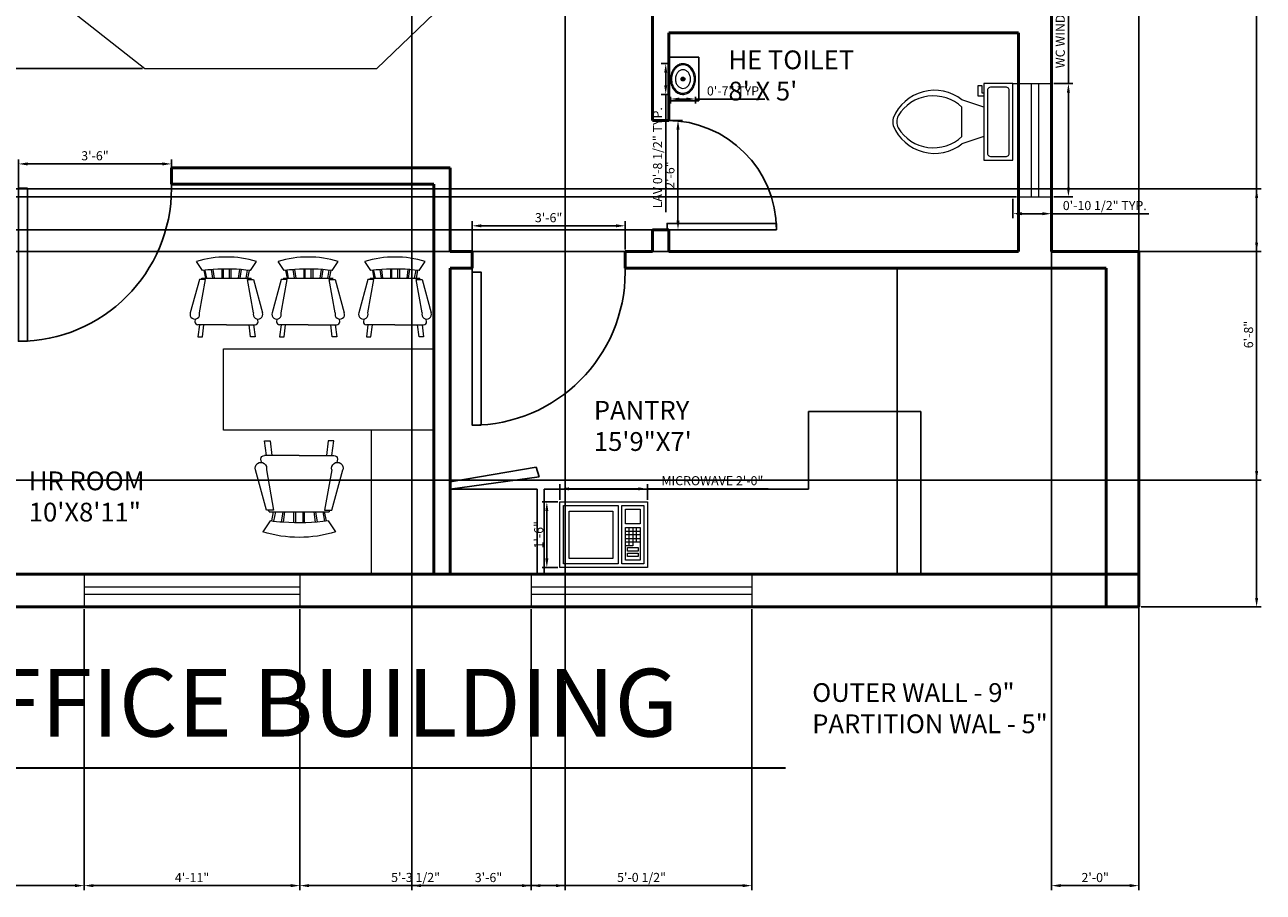
# Model space of a CAD drawing. Units: inches. Extents: x -4852 to -4300, y 4342 to 5059.
# Tile 2 of 4: x -4640 to -4300, y 4342 to 4580. Entities that reach past the tile are written whole.
import ezdxf

# ---------------------------------------------------------------- set-up
doc = ezdxf.new("R2010")
doc.units = ezdxf.units.IN
for name, color, linetype, lineweight in [('A-ANNO-DIMS', 2, 'Continuous', 18), ('A-ANNO-TEXT', 7, 'Continuous', 18), ('A-ANNO-TITL', 7, 'Continuous', 35), ('A-AREA-IDEN', 7, 'Continuous', 18), ('A-DOOR', 4, 'Continuous', 25), ('A-EQPM', 8, 'Continuous', 18), ('A-FLOR-CASE', 9, 'Continuous', 25), ('A-FLOR-FIXT', 9, 'Continuous', 18), ('A-FURN', 8, 'Continuous', 18), ('A-GLAZ', 4, 'Continuous', 18), ('A-WALL', 7, 'Continuous', 50)]:
    doc.layers.add(name, color=color, linetype=linetype, lineweight=lineweight)
doc.styles.get("Standard").update_dxf_attribs({"font": 'arial.ttf'})
doc.dimstyles.new('ISO-25', dxfattribs={"dimtxt": 2.5, "dimasz": 2.5, "dimexe": 1.25, "dimexo": 0.625, "dimtad": 1, "dimdec": 0, "dimlunit": 3, "dimtxsty": 'Standard', "dimcen": 2.5, "dimadec": 0, "dimazin": 0, "dimtfac": 1, "dimtdec": 0, "dimtmove": 0, "dimatfit": 3, "dimfxl": 1, "dimarcsym": 0})

# ---------------------------------------------------------------- blocks, each defined once
blk = doc.blocks.new('*U2')
for p, q in [((0, 0), (0, -100)), ((750, 0), (750, -100))]:
    blk.add_line(p, q)
blk.add_lwpolyline([(0, 0), (0, 750), (43.75, 750), (43.75, 0)], close=True)
blk.add_arc((0, 0), 750, 0, 90)
blk = doc.blocks.new('Microwave')
for p, q in [((19, 7), (19, 11)), ((20, 11), (20, 7)), ((21, 7), (21, 11)), ((18, 10), (22, 10)), ((22, 9), (18, 9)), ((18, 8), (22, 8)), ((22, 7), (18, 7)), ((19, 6), (19, 7)), ((20, 7), (20, 6)), ((20, 6), (18, 6))]:
    blk.add_line(p, q)
for points in [[(0, 0), (0, 18), (24, 18), (24, 0)], [(1, 1), (1, 17), (16, 17), (16, 1)], [(17, 1), (17, 17), (23, 17), (23, 1)], [(2.5, 2.5), (2.5, 15.5), (14.5, 15.5), (14.5, 2.5)], [(18, 12), (18, 16), (22, 16), (22, 12)], [(18, 2), (18, 11), (22, 11), (22, 2)], [(18.5, 4.5), (18.5, 5.5), (21.5, 5.5), (21.5, 4.5)], [(18.5, 3), (18.5, 4), (21.5, 4), (21.5, 3)]]:
    blk.add_lwpolyline(points, close=True)
blk = doc.blocks.new('Toilet - top')
for p, q in [((9.5, -6), (9.5, -2)), ((-10, -8.5), (-8, -8.5)), ((-10, -9.5), (-10, -8.5)), ((-7, -9.5), (-10, -9.5)), ((-8, -8.5), (-8, -8)), ((-7, -8), (-7, -9.5)), ((-4, -8), (-6, -14)), ((4, -8), (6, -14)), ((4, -14), (-4, -14))]:
    blk.add_line(p, q)
blk.add_lwpolyline([(10.5, -8), (10.5, 0), (-10.5, 0), (-10.5, -8)], close=True)
for points in [[(-9.5, -2), (-9.5, -6)], [(8.5, -1), (-8.5, -1)], [(-8.5, -7), (8.5, -7)]]:
    blk.add_lwpolyline(points)
for centre, radius, start, end in [((-8.62, -1.88), 0.884, 81.8699, 188.1301), ((8.62, -1.88), 0.884, 351.8699, 98.1301), ((-8.62, -6.12), 0.884, 171.8699, 278.1301), ((8.62, -6.12), 0.884, 261.8699, 8.1301), ((3.52, -21.58), 12.17, 141.4691, 247.9714), ((4.2, -21.82), 11.33, 136.3677, 238.9468), ((-3.52, -21.58), 12.17, 292.0284, 38.5307), ((-4.2, -21.82), 11.33, 301.053, 43.6321), ((0, -27.88), 4, 245.7318, 294.2682), ((0, -29), 4, 254.8605, 285.1395)]:
    blk.add_arc(centre, radius, start, end)
blk = doc.blocks.new('Sink - Oval top')
for p, q in [((-1, 0), (1, 0)), ((0, 1), (0, -1))]:
    blk.add_line(p, q)
for points in [[(-12.23, 0.39, 0.117634), (-11.46, -3.36, 0.104469), (-8.88, -6.8, 0.090016), (-5.08, -9.07, 0.08192), (-0.32, -10.02, 0.08192), (4.49, -9.38, 0.090016), (8.42, -7.36, 0.104469), (11.22, -4.09, 0.117634), (12.23, -0.39, 0.117634), (11.46, 3.36, 0.104469), (8.88, 6.8, 0.090016), (5.08, 9.07, 0.08192), (0.32, 10.02, 0.08192), (-4.49, 9.38, 0.090016), (-8.42, 7.36, 0.104469), (-11.22, 4.09, 0.117634)], [(-11.29, 0.16, 0.118622), (-10.52, -3.25, 0.104678), (-8.07, -6.36, 0.089562), (-4.54, -8.37, 0.081185), (-0.13, -9.15, 0.081185), (4.3, -8.49, 0.089562), (7.89, -6.58, 0.104678), (10.42, -3.55, 0.118622), (11.29, -0.16, 0.118622), (10.52, 3.25, 0.104678), (8.07, 6.36, 0.089562), (4.54, 8.37, 0.081185), (0.13, 9.15, 0.081185), (-4.3, 8.49, 0.089562), (-7.89, 6.58, 0.104678), (-10.42, 3.55, 0.118622)], [(-7.42, 0.08, 0.118283), (-6.91, -2.17, 0.104607), (-5.29, -4.21, 0.089718), (-2.97, -5.53, 0.081436), (-0.07, -6.04, 0.081436), (2.84, -5.59, 0.089718), (5.2, -4.33, 0.104607), (6.86, -2.32, 0.118283), (7.42, -0.08, 0.118283), (6.91, 2.17, 0.104607), (5.29, 4.21, 0.089718), (2.97, 5.53, 0.081436), (0.07, 6.04, 0.081436), (-2.84, 5.59, 0.089718), (-5.2, 4.33, 0.104607), (-6.86, 2.32, 0.118283)]]:
    blk.add_lwpolyline(points, format="xyb", close=True)
for radius in [1.5, 1]:
    blk.add_circle((0, 0), radius)
blk = doc.blocks.new('Chair - Rocking')
for p, q in [((-8, -4.5), (-10, -1.5)), ((8, -4.5), (10, -1.5)), ((-7.5, -4.5), (-7, -7)), ((-6.5, -7), (-7.02225, -4.43)), ((-4.5, -7), (-4.96674, -4.19951)), ((-4, -7), (-4.40532, -4.16272)), ((-1.5, -4.05012), (-1.5, -7)), ((-1, -7), (-1, -4.05012)), ((1, -7), (1, -4.04655)), ((1.5, -4.05012), (1.5, -7)), ((4, -7), (4.40187, -4.18694)), ((4.5, -7), (4.96761, -4.19437)), ((6.5, -7), (7, -4.4057)), ((7.5, -4.5), (7, -7)), ((-9, -7.5), (-12, -18.49999)), ((-7, -7.5), (-9, -7.5)), ((-9, -18.49999), (-7, -7.5)), ((-8.23428, -6.99939), (-8.3093, -7.47958)), ((-8.23041, -7), (8.23915, -7)), ((7, -7.5), (9, -7.5)), ((9, -18.49999), (7, -7.5)), ((8.31071, -7.48854), (8.23449, -7.00073)), ((9, -7.5), (12, -18.49999)), ((-10.36644, -20.64523), (-10.5, -21.49999)), ((-9, -22.49999), (-9.5, -26.49999)), ((0, -22.49999), (-9.5, -22.49999)), ((-8, -26.49999), (-7.5, -22.49999)), ((0, -22.49999), (9.5, -22.49999)), ((8, -26.49999), (7.5, -22.49999)), ((9, -22.49999), (9.5, -26.49999)), ((10.5, -21.49999), (10.3575, -20.58798)), ((-9.5, -26.49999), (-8, -26.49999)), ((9.5, -26.49999), (8, -26.49999))]:
    blk.add_line(p, q)
for centre, radius, start, end in [((0, -34.08333), 34.08333, 72.93847, 107.0615), ((0, -68.25004), 64.25, 93.92211, 97.15267), ((0, -68.25004), 64.25, 82.84733, 93.92211), ((-10.5, -18.99999), 1.58114, 161.5651, 18.43495), ((10.5, -18.99999), 1.58114, 161.5651, 18.43495), ((-9.5, -21.49999), 1, 180, 270), ((9.5, -21.49999), 1, 270, 0)]:
    blk.add_arc(centre, radius, start, end)
blk = doc.blocks.new('*D9')
at = {"layer": 'A-ANNO-DIMS', "color": 0, "lineweight": -2, "transparency": 16777216}
for p, q in [((-4641.4, 4535.4), (-4641.4, 4542.7)), ((-4638.9, 4541.45), (-4601.9, 4541.45)), ((-4599.4, 4536.5), (-4599.4, 4542.7))]:
    blk.add_line(p, q, dxfattribs=at)
at = {"layer": 'A-ANNO-DIMS', "color": 0, "transparency": 16777216}
for points in [[(-4638.9, 4541.87), (-4638.9, 4541.04), (-4641.4, 4541.45)], [(-4601.9, 4541.87), (-4601.9, 4541.04), (-4599.4, 4541.45)]]:
    blk.add_solid(points, dxfattribs=at)
at = {"layer": 'Defpoints', "color": 0, "transparency": 16777216}
for p in [(-4599.4, 4541.45), (-4641.4, 4534.78), (-4599.4, 4535.88)]:
    blk.add_point(p, dxfattribs=at)
at = {"layer": 'A-ANNO-DIMS', "color": 0, "transparency": 16777216, "insert": (-4620.4, 4543.36), "char_height": 2.5, "attachment_point": 5}
blk.add_mtext('3\'-6"', dxfattribs=at)
blk = doc.blocks.new('*D10')
at = {"layer": 'A-ANNO-DIMS', "color": 0, "lineweight": -2, "transparency": 16777216}
for p, q in [((-4516.9, 4515.75), (-4516.9, 4525.72)), ((-4477.4, 4524.47), (-4514.4, 4524.47)), ((-4474.9, 4518), (-4474.9, 4525.72))]:
    blk.add_line(p, q, dxfattribs=at)
at = {"layer": 'A-ANNO-DIMS', "color": 0, "transparency": 16777216}
for points in [[(-4514.4, 4524.89), (-4514.4, 4524.06), (-4516.9, 4524.47)], [(-4477.4, 4524.89), (-4477.4, 4524.06), (-4474.9, 4524.47)]]:
    blk.add_solid(points, dxfattribs=at)
at = {"layer": 'Defpoints', "color": 0, "transparency": 16777216}
for p in [(-4516.9, 4524.47), (-4474.9, 4517.38), (-4516.9, 4515.13)]:
    blk.add_point(p, dxfattribs=at)
at = {"layer": 'A-ANNO-DIMS', "color": 0, "transparency": 16777216, "insert": (-4495.9, 4526.38), "char_height": 2.5, "attachment_point": 5}
blk.add_mtext('3\'-6"', dxfattribs=at)
blk = doc.blocks.new('*D11')
at = {"layer": 'A-ANNO-DIMS', "color": 0, "lineweight": -2, "transparency": 16777216}
for p, q in [((-4466.77, 4553.38), (-4459.14, 4553.38)), ((-4460.39, 4550.88), (-4460.39, 4525.88)), ((-4466.77, 4523.38), (-4459.14, 4523.38))]:
    blk.add_line(p, q, dxfattribs=at)
at = {"layer": 'A-ANNO-DIMS', "color": 0, "transparency": 16777216}
for points in [[(-4460.81, 4550.88), (-4459.97, 4550.88), (-4460.39, 4553.38)], [(-4460.81, 4525.88), (-4459.97, 4525.88), (-4460.39, 4523.38)]]:
    blk.add_solid(points, dxfattribs=at)
at = {"layer": 'Defpoints', "color": 0, "transparency": 16777216}
for p in [(-4467.4, 4553.38), (-4467.4, 4523.38), (-4460.39, 4523.38)]:
    blk.add_point(p, dxfattribs=at)
at = {"layer": 'A-ANNO-DIMS', "color": 0, "transparency": 16777216, "insert": (-4462.29, 4538.38), "char_height": 2.5, "attachment_point": 5, "rotation": 90}
blk.add_mtext('2\'-6"', dxfattribs=at)
blk = doc.blocks.new('VANITY-COMPACT')
for p, q in [((8.23, 12.02), (0, 12.02)), ((8.23, 0), (8.23, 12.02)), ((0, 0), (8.23, 0))]:
    blk.add_line(p, q)
blk = doc.blocks.new('WIN-RESTROOM')
for p, q in [((0, 31.05), (10.57, 31.05)), ((5.07, 0), (5.07, 31.05)), ((7.07, 0), (7.07, 31.05)), ((1.57, 0), (10.57, 0))]:
    blk.add_line(p, q)
blk = doc.blocks.new('*D31')
at = {"layer": 'A-ANNO-DIMS', "color": 0, "lineweight": -2, "transparency": 16777216}
for p, q in [((-4463.11, 4568.96), (-4465.01, 4568.96)), ((-4463.76, 4566.46), (-4463.76, 4563.02)), ((-4463.11, 4560.52), (-4465.01, 4560.52)), ((-4463.76, 4560.52), (-4463.76, 4528.25))]:
    blk.add_line(p, q, dxfattribs=at)
at = {"layer": 'A-ANNO-DIMS', "color": 0, "transparency": 16777216}
for points in [[(-4464.17, 4566.46), (-4463.34, 4566.46), (-4463.76, 4568.96)], [(-4464.17, 4563.02), (-4463.34, 4563.02), (-4463.76, 4560.52)]]:
    blk.add_solid(points, dxfattribs=at)
at = {"layer": 'Defpoints', "color": 0, "transparency": 16777216}
for p in [(-4462.49, 4568.96), (-4463.76, 4560.52), (-4462.49, 4560.52)]:
    blk.add_point(p, dxfattribs=at)
at = {"layer": 'A-ANNO-DIMS', "color": 0, "transparency": 16777216, "insert": (-4465.67, 4543.14), "char_height": 2.5, "attachment_point": 5, "rotation": 90}
blk.add_mtext('LAV 0\'-8 1/2" TYP.', dxfattribs=at)
blk = doc.blocks.new('*D32')
at = {"layer": 'A-ANNO-DIMS', "color": 0, "lineweight": -2, "transparency": 16777216}
for p, q in [((-4462.49, 4559.9), (-4462.49, 4558.01)), ((-4459.99, 4559.26), (-4458.07, 4559.26)), ((-4455.57, 4559.9), (-4455.57, 4558.01)), ((-4455.57, 4559.26), (-4436.58, 4559.26))]:
    blk.add_line(p, q, dxfattribs=at)
at = {"layer": 'A-ANNO-DIMS', "color": 0, "transparency": 16777216}
for points in [[(-4459.99, 4559.67), (-4459.99, 4558.84), (-4462.49, 4559.26)], [(-4458.07, 4559.67), (-4458.07, 4558.84), (-4455.57, 4559.26)]]:
    blk.add_solid(points, dxfattribs=at)
at = {"layer": 'Defpoints', "color": 0, "transparency": 16777216}
for p in [(-4462.49, 4560.52), (-4455.57, 4560.52), (-4455.57, 4559.26)]:
    blk.add_point(p, dxfattribs=at)
at = {"layer": 'A-ANNO-DIMS', "color": 0, "transparency": 16777216, "insert": (-4444.82, 4561.16), "char_height": 2.5, "attachment_point": 5}
blk.add_mtext('0\'-7" TYP.', dxfattribs=at)
blk = doc.blocks.new('*D35')
at = {"layer": 'A-ANNO-DIMS', "color": 0, "lineweight": -2, "transparency": 16777216}
for p, q in [((-4353.24, 4563.5), (-4353.24, 4605.68)), ((-4357.27, 4563.5), (-4351.99, 4563.5)), ((-4353.24, 4534.95), (-4353.24, 4561)), ((-4357.27, 4532.45), (-4351.99, 4532.45))]:
    blk.add_line(p, q, dxfattribs=at)
at = {"layer": 'A-ANNO-DIMS', "color": 0, "transparency": 16777216}
for points in [[(-4353.66, 4561), (-4352.83, 4561), (-4353.24, 4563.5)], [(-4353.66, 4534.95), (-4352.83, 4534.95), (-4353.24, 4532.45)]]:
    blk.add_solid(points, dxfattribs=at)
at = {"layer": 'Defpoints', "color": 0, "transparency": 16777216}
for p in [(-4357.9, 4563.5), (-4353.24, 4563.5), (-4357.9, 4532.45)]:
    blk.add_point(p, dxfattribs=at)
at = {"layer": 'A-ANNO-DIMS', "color": 0, "transparency": 16777216, "insert": (-4355.16, 4585.84), "char_height": 2.5, "attachment_point": 5, "rotation": 90}
blk.add_mtext('WC WINDOW 2\'-7" TYP.', dxfattribs=at)
blk = doc.blocks.new('*D36')
at = {"layer": 'A-ANNO-DIMS', "color": 0, "lineweight": -2, "transparency": 16777216}
for p, q in [((-4368.47, 4531.83), (-4368.47, 4526.55)), ((-4357.9, 4531.83), (-4357.9, 4526.55)), ((-4365.97, 4527.8), (-4360.4, 4527.8)), ((-4357.9, 4527.8), (-4331.14, 4527.8))]:
    blk.add_line(p, q, dxfattribs=at)
at = {"layer": 'A-ANNO-DIMS', "color": 0, "transparency": 16777216}
for points in [[(-4365.97, 4528.21), (-4365.97, 4527.38), (-4368.47, 4527.8)], [(-4360.4, 4528.21), (-4360.4, 4527.38), (-4357.9, 4527.8)]]:
    blk.add_solid(points, dxfattribs=at)
at = {"layer": 'Defpoints', "color": 0, "transparency": 16777216}
for p in [(-4368.47, 4532.45), (-4357.9, 4532.45), (-4357.9, 4527.8)]:
    blk.add_point(p, dxfattribs=at)
at = {"layer": 'A-ANNO-DIMS', "color": 0, "transparency": 16777216, "insert": (-4343.27, 4529.71), "char_height": 2.5, "attachment_point": 5}
blk.add_mtext('0\'-10 1/2" TYP.', dxfattribs=at)
blk = doc.blocks.new('*D37')
at = {"layer": 'A-ANNO-DIMS', "color": 0, "lineweight": -2, "transparency": 16777216}
for p, q in [((-4492.79, 4449.32), (-4492.79, 4453.54)), ((-4468.79, 4449.32), (-4468.79, 4453.54)), ((-4490.29, 4452.29), (-4471.29, 4452.29)), ((-4468.79, 4452.29), (-4435.61, 4452.29))]:
    blk.add_line(p, q, dxfattribs=at)
at = {"layer": 'A-ANNO-DIMS', "color": 0, "transparency": 16777216}
for points in [[(-4490.29, 4452.71), (-4490.29, 4451.88), (-4492.79, 4452.29)], [(-4471.29, 4452.71), (-4471.29, 4451.88), (-4468.79, 4452.29)]]:
    blk.add_solid(points, dxfattribs=at)
at = {"layer": 'Defpoints', "color": 0, "transparency": 16777216}
for p in [(-4468.79, 4452.29), (-4492.79, 4448.69), (-4468.79, 4448.69)]:
    blk.add_point(p, dxfattribs=at)
at = {"layer": 'A-ANNO-DIMS', "color": 0, "transparency": 16777216, "insert": (-4450.95, 4454.21), "char_height": 2.5, "attachment_point": 5}
blk.add_mtext('MICROWAVE 2\'-0"', dxfattribs=at)
blk = doc.blocks.new('*D38')
at = {"layer": 'A-ANNO-DIMS', "color": 0, "lineweight": -2, "transparency": 16777216}
for p, q in [((-4493.41, 4448.69), (-4497.64, 4448.69)), ((-4496.39, 4433.19), (-4496.39, 4446.19)), ((-4493.41, 4430.69), (-4497.64, 4430.69))]:
    blk.add_line(p, q, dxfattribs=at)
at = {"layer": 'A-ANNO-DIMS', "color": 0, "transparency": 16777216}
for points in [[(-4496.8, 4446.19), (-4495.97, 4446.19), (-4496.39, 4448.69)], [(-4496.8, 4433.19), (-4495.97, 4433.19), (-4496.39, 4430.69)]]:
    blk.add_solid(points, dxfattribs=at)
at = {"layer": 'Defpoints', "color": 0, "transparency": 16777216}
for p in [(-4496.39, 4448.69), (-4492.79, 4448.69), (-4492.79, 4430.69)]:
    blk.add_point(p, dxfattribs=at)
at = {"layer": 'A-ANNO-DIMS', "color": 0, "transparency": 16777216, "insert": (-4498.29, 4439.69), "char_height": 2.5, "attachment_point": 5, "rotation": 90}
blk.add_mtext('1\'-6"', dxfattribs=at)
blk = doc.blocks.new('*D40')
at = {"layer": 'A-ANNO-DIMS', "color": 0, "lineweight": -2, "transparency": 16777216}
for p, q in [((-4333.27, 5021.38), (-4300.34, 5021.38)), ((-4301.59, 4422.38), (-4301.59, 5018.88)), ((-4333.27, 4419.88), (-4300.34, 4419.88))]:
    blk.add_line(p, q, dxfattribs=at)
at = {"layer": 'A-ANNO-DIMS', "color": 0, "transparency": 16777216}
for points in [[(-4302.01, 5018.88), (-4301.17, 5018.88), (-4301.59, 5021.38)], [(-4302.01, 4422.38), (-4301.17, 4422.38), (-4301.59, 4419.88)]]:
    blk.add_solid(points, dxfattribs=at)
at = {"layer": 'Defpoints', "color": 0, "transparency": 16777216}
for p in [(-4333.9, 5021.38), (-4301.59, 5021.38), (-4333.9, 4419.88)]:
    blk.add_point(p, dxfattribs=at)
at = {"layer": 'A-ANNO-DIMS', "color": 0, "transparency": 16777216, "insert": (-4303.51, 4720.63), "char_height": 2.5, "attachment_point": 5, "rotation": 90}
blk.add_mtext('50\'-1 1/2"', dxfattribs=at)
blk = doc.blocks.new('*D43')
at = {"layer": 'A-ANNO-DIMS', "color": 0, "lineweight": -2, "transparency": 16777216}
for p, q in [((-4357.9, 4705.75), (-4357.9, 4342.18)), ((-4333.9, 4705.75), (-4333.9, 4342.18)), ((-4355.4, 4343.43), (-4336.4, 4343.43))]:
    blk.add_line(p, q, dxfattribs=at)
at = {"layer": 'A-ANNO-DIMS', "color": 0, "transparency": 16777216}
for points in [[(-4355.4, 4343.85), (-4355.4, 4343.01), (-4357.9, 4343.43)], [(-4336.4, 4343.85), (-4336.4, 4343.01), (-4333.9, 4343.43)]]:
    blk.add_solid(points, dxfattribs=at)
at = {"layer": 'Defpoints', "color": 0, "transparency": 16777216}
for p in [(-4357.9, 4706.38), (-4333.9, 4706.38), (-4333.9, 4343.43)]:
    blk.add_point(p, dxfattribs=at)
at = {"layer": 'A-ANNO-DIMS', "color": 0, "transparency": 16777216, "insert": (-4345.9, 4345.33), "char_height": 2.5, "attachment_point": 5}
blk.add_mtext('2\'-0"', dxfattribs=at)
blk = doc.blocks.new('*D44')
at = {"layer": 'A-ANNO-DIMS', "color": 0, "lineweight": -2, "transparency": 16777216}
for p, q in [((-4357.27, 4706.38), (-4300.34, 4706.38)), ((-4301.59, 4519.88), (-4301.59, 4703.88)), ((-4357.27, 4517.38), (-4300.34, 4517.38))]:
    blk.add_line(p, q, dxfattribs=at)
at = {"layer": 'A-ANNO-DIMS', "color": 0, "transparency": 16777216}
for points in [[(-4302.01, 4703.88), (-4301.17, 4703.88), (-4301.59, 4706.38)], [(-4302.01, 4519.88), (-4301.17, 4519.88), (-4301.59, 4517.38)]]:
    blk.add_solid(points, dxfattribs=at)
at = {"layer": 'Defpoints', "color": 0, "transparency": 16777216}
for p in [(-4357.9, 4706.38), (-4301.59, 4706.38), (-4357.9, 4517.38)]:
    blk.add_point(p, dxfattribs=at)
at = {"layer": 'A-ANNO-DIMS', "color": 0, "transparency": 16777216, "insert": (-4303.49, 4611.88), "char_height": 2.5, "attachment_point": 5, "rotation": 90}
blk.add_mtext('15\'-9"', dxfattribs=at)
blk = doc.blocks.new('*D54')
at = {"layer": 'A-ANNO-DIMS', "color": 0, "lineweight": -2, "transparency": 16777216}
for p, q in [((-4813.9, 4419.25), (-4813.9, 4342.18)), ((-4623.35, 4419.25), (-4623.35, 4342.18)), ((-4811.4, 4343.43), (-4625.85, 4343.43))]:
    blk.add_line(p, q, dxfattribs=at)
at = {"layer": 'A-ANNO-DIMS', "color": 0, "transparency": 16777216}
for points in [[(-4811.4, 4343.85), (-4811.4, 4343.01), (-4813.9, 4343.43)], [(-4625.85, 4343.85), (-4625.85, 4343.01), (-4623.35, 4343.43)]]:
    blk.add_solid(points, dxfattribs=at)
at = {"layer": 'Defpoints', "color": 0, "transparency": 16777216}
for p in [(-4813.9, 4419.88), (-4623.35, 4419.88), (-4623.35, 4343.43)]:
    blk.add_point(p, dxfattribs=at)
at = {"layer": 'A-ANNO-DIMS', "color": 0, "transparency": 16777216, "insert": (-4718.62, 4345.35), "char_height": 2.5, "attachment_point": 5}
blk.add_mtext('15\'-10 1/2"', dxfattribs=at)
blk = doc.blocks.new('*D55')
at = {"layer": 'A-ANNO-DIMS', "color": 0, "lineweight": -2, "transparency": 16777216}
for p, q in [((-4623.35, 4419.25), (-4623.35, 4342.18)), ((-4564.15, 4419.25), (-4564.15, 4342.18)), ((-4620.85, 4343.43), (-4566.65, 4343.43))]:
    blk.add_line(p, q, dxfattribs=at)
at = {"layer": 'A-ANNO-DIMS', "color": 0, "transparency": 16777216}
for points in [[(-4620.85, 4343.85), (-4620.85, 4343.01), (-4623.35, 4343.43)], [(-4566.65, 4343.85), (-4566.65, 4343.01), (-4564.15, 4343.43)]]:
    blk.add_solid(points, dxfattribs=at)
at = {"layer": 'Defpoints', "color": 0, "transparency": 16777216}
for p in [(-4623.35, 4419.88), (-4564.15, 4419.88), (-4564.15, 4343.43)]:
    blk.add_point(p, dxfattribs=at)
at = {"layer": 'A-ANNO-DIMS', "color": 0, "transparency": 16777216, "insert": (-4593.75, 4345.31), "char_height": 2.5, "attachment_point": 5}
blk.add_mtext('4\'-11"', dxfattribs=at)
blk = doc.blocks.new('*D56')
at = {"layer": 'A-ANNO-DIMS', "color": 0, "lineweight": -2, "transparency": 16777216}
for p, q in [((-4564.15, 4419.25), (-4564.15, 4342.18)), ((-4500.68, 4419.25), (-4500.68, 4342.18)), ((-4561.65, 4343.43), (-4503.18, 4343.43))]:
    blk.add_line(p, q, dxfattribs=at)
at = {"layer": 'A-ANNO-DIMS', "color": 0, "transparency": 16777216}
for points in [[(-4561.65, 4343.85), (-4561.65, 4343.01), (-4564.15, 4343.43)], [(-4503.18, 4343.85), (-4503.18, 4343.01), (-4500.68, 4343.43)]]:
    blk.add_solid(points, dxfattribs=at)
at = {"layer": 'Defpoints', "color": 0, "transparency": 16777216}
for p in [(-4564.15, 4419.88), (-4500.68, 4419.88), (-4500.68, 4343.43)]:
    blk.add_point(p, dxfattribs=at)
at = {"layer": 'A-ANNO-DIMS', "color": 0, "transparency": 16777216, "insert": (-4532.41, 4345.35), "char_height": 2.5, "attachment_point": 5}
blk.add_mtext('5\'-3 1/2"', dxfattribs=at)
blk = doc.blocks.new('*D57')
at = {"layer": 'A-ANNO-DIMS', "color": 0, "lineweight": -2, "transparency": 16777216}
for p, q in [((-4500.68, 4419.25), (-4500.68, 4342.18)), ((-4440.12, 4419.25), (-4440.12, 4342.18)), ((-4498.18, 4343.43), (-4442.62, 4343.43))]:
    blk.add_line(p, q, dxfattribs=at)
at = {"layer": 'A-ANNO-DIMS', "color": 0, "transparency": 16777216}
for points in [[(-4498.18, 4343.85), (-4498.18, 4343.01), (-4500.68, 4343.43)], [(-4442.62, 4343.85), (-4442.62, 4343.01), (-4440.12, 4343.43)]]:
    blk.add_solid(points, dxfattribs=at)
at = {"layer": 'Defpoints', "color": 0, "transparency": 16777216}
for p in [(-4500.68, 4419.88), (-4440.12, 4419.88), (-4440.12, 4343.43)]:
    blk.add_point(p, dxfattribs=at)
at = {"layer": 'A-ANNO-DIMS', "color": 0, "transparency": 16777216, "insert": (-4470.4, 4345.35), "char_height": 2.5, "attachment_point": 5}
blk.add_mtext('5\'-0 1/2"', dxfattribs=at)
blk = doc.blocks.new('*D59')
at = {"layer": 'A-ANNO-DIMS', "color": 0, "lineweight": -2, "transparency": 16777216}
for p, q in [((-4533.4, 4761.25), (-4533.4, 4342.18)), ((-4491.4, 4761.25), (-4491.4, 4342.18)), ((-4530.9, 4343.43), (-4493.9, 4343.43))]:
    blk.add_line(p, q, dxfattribs=at)
at = {"layer": 'A-ANNO-DIMS', "color": 0, "transparency": 16777216}
for points in [[(-4530.9, 4343.85), (-4530.9, 4343.01), (-4533.4, 4343.43)], [(-4493.9, 4343.85), (-4493.9, 4343.01), (-4491.4, 4343.43)]]:
    blk.add_solid(points, dxfattribs=at)
at = {"layer": 'Defpoints', "color": 0, "transparency": 16777216}
for p in [(-4533.4, 4761.88), (-4491.4, 4761.88), (-4491.4, 4343.43)]:
    blk.add_point(p, dxfattribs=at)
at = {"layer": 'A-ANNO-DIMS', "color": 0, "transparency": 16777216, "insert": (-4512.4, 4345.33), "char_height": 2.5, "attachment_point": 5}
blk.add_mtext('3\'-6"', dxfattribs=at)
blk = doc.blocks.new('*D61')
at = {"layer": 'A-ANNO-DIMS', "color": 0, "lineweight": -2, "transparency": 16777216}
for p, q in [((-4635.56, 4696.34), (-4847.46, 4696.34)), ((-4846.21, 4693.84), (-4846.21, 4570.1)), ((-4607.33, 4567.6), (-4847.46, 4567.6))]:
    blk.add_line(p, q, dxfattribs=at)
at = {"layer": 'A-ANNO-DIMS', "color": 0, "transparency": 16777216}
for points in [[(-4846.63, 4693.84), (-4845.79, 4693.84), (-4846.21, 4696.34)], [(-4846.63, 4570.1), (-4845.79, 4570.1), (-4846.21, 4567.6)]]:
    blk.add_solid(points, dxfattribs=at)
at = {"layer": 'Defpoints', "color": 0, "transparency": 16777216}
for p in [(-4634.93, 4696.34), (-4846.21, 4567.6), (-4606.71, 4567.6)]:
    blk.add_point(p, dxfattribs=at)
at = {"layer": 'A-ANNO-DIMS', "color": 0, "transparency": 16777216, "insert": (-4848.13, 4631.97), "char_height": 2.5, "attachment_point": 5, "rotation": 90}
blk.add_mtext('10\'-8 1/2"', dxfattribs=at)
blk = doc.blocks.new('*D63')
at = {"layer": 'A-ANNO-DIMS', "color": 0, "lineweight": -2, "transparency": 16777216}
for p, q in [((-4757.25, 4534.6), (-4300.34, 4534.6)), ((-4301.59, 4457.19), (-4301.59, 4532.1)), ((-4757.25, 4454.69), (-4300.34, 4454.69))]:
    blk.add_line(p, q, dxfattribs=at)
at = {"layer": 'A-ANNO-DIMS', "color": 0, "transparency": 16777216}
for points in [[(-4302.01, 4532.1), (-4301.17, 4532.1), (-4301.59, 4534.6)], [(-4302.01, 4457.19), (-4301.17, 4457.19), (-4301.59, 4454.69)]]:
    blk.add_solid(points, dxfattribs=at)
at = {"layer": 'Defpoints', "color": 0, "transparency": 16777216}
for p in [(-4757.87, 4534.6), (-4301.59, 4534.6), (-4757.87, 4454.69)]:
    blk.add_point(p, dxfattribs=at)
at = {"layer": 'A-ANNO-DIMS', "color": 0, "transparency": 16777216, "insert": (-4303.49, 4494.64), "char_height": 2.5, "attachment_point": 5, "rotation": 90}
blk.add_mtext('6\'-8"', dxfattribs=at)
blk = doc.blocks.new('*D64')
at = {"layer": 'A-ANNO-DIMS', "color": 0, "lineweight": -2, "transparency": 16777216}
for p, q in [((-4846.21, 4525.88), (-4846.21, 4536.27)), ((-4463.52, 4523.38), (-4847.46, 4523.38)), ((-4846.21, 4517.38), (-4846.21, 4523.38)), ((-4463.52, 4517.38), (-4847.46, 4517.38)), ((-4846.21, 4514.88), (-4846.21, 4512.38))]:
    blk.add_line(p, q, dxfattribs=at)
at = {"layer": 'A-ANNO-DIMS', "color": 0, "transparency": 16777216}
for points in [[(-4846.63, 4525.88), (-4845.79, 4525.88), (-4846.21, 4523.38)], [(-4846.63, 4514.88), (-4845.79, 4514.88), (-4846.21, 4517.38)]]:
    blk.add_solid(points, dxfattribs=at)
at = {"layer": 'Defpoints', "color": 0, "transparency": 16777216}
for p in [(-4846.21, 4523.38), (-4462.9, 4523.38), (-4462.9, 4517.38)]:
    blk.add_point(p, dxfattribs=at)
at = {"layer": 'A-ANNO-DIMS', "color": 0, "transparency": 16777216, "insert": (-4848.11, 4532.33), "char_height": 2.5, "attachment_point": 5, "rotation": 90}
blk.add_mtext('0\'-6"', dxfattribs=at)
blk = doc.blocks.new('*D65')
at = {"layer": 'A-ANNO-DIMS', "color": 0, "lineweight": -2, "transparency": 16777216}
for p, q in [((-4367.52, 4532.45), (-4847.46, 4532.45)), ((-4846.21, 4519.88), (-4846.21, 4529.95)), ((-4367.52, 4517.38), (-4847.46, 4517.38))]:
    blk.add_line(p, q, dxfattribs=at)
at = {"layer": 'A-ANNO-DIMS', "color": 0, "transparency": 16777216}
for points in [[(-4846.63, 4529.95), (-4845.79, 4529.95), (-4846.21, 4532.45)], [(-4846.63, 4519.88), (-4845.79, 4519.88), (-4846.21, 4517.38)]]:
    blk.add_solid(points, dxfattribs=at)
at = {"layer": 'Defpoints', "color": 0, "transparency": 16777216}
for p in [(-4846.21, 4532.45), (-4366.9, 4532.45), (-4366.9, 4517.38)]:
    blk.add_point(p, dxfattribs=at)
at = {"layer": 'A-ANNO-DIMS', "color": 0, "transparency": 16777216, "insert": (-4848.11, 4524.92), "char_height": 2.5, "attachment_point": 5, "rotation": 90}
blk.add_mtext('1\'-3"', dxfattribs=at)

msp = doc.modelspace()

# ---------------------------------------------------------------- linework, layer by layer
at = {"layer": 'A-ANNO-TITL'}
msp.add_line((-4794.71, 4375.74), (-4430.92, 4375.74), dxfattribs=at)
at = {"layer": 'A-FLOR-CASE'}
for p, q in [((-4400.28, 4512.88), (-4400.28, 4428.88)), ((-4393.78, 4473.51), (-4424.55, 4473.51)), ((-4424.55, 4473.51), (-4424.55, 4452.2)), ((-4393.78, 4428.88), (-4393.78, 4473.51)), ((-4499.31, 4458.29), (-4522.9, 4454.2)), ((-4498.45, 4455.6), (-4499.31, 4458.29)), ((-4522.9, 4452.2), (-4498.45, 4455.6)), ((-4499.08, 4452.2), (-4522.9, 4452.2)), ((-4499.08, 4452.2), (-4499.08, 4428.88)), ((-4424.55, 4452.2), (-4497.08, 4452.2)), ((-4497.08, 4452.2), (-4497.08, 4428.88))]:
    msp.add_line(p, q, dxfattribs=at)
at = {"layer": 'A-FURN'}
for p, q in [((-4634.93, 4589.86), (-4606.71, 4567.6)), ((-4543.07, 4567.6), (-4519.98, 4589.79)), ((-4606.71, 4567.6), (-4543.07, 4567.6)), ((-4544.64, 4468.4), (-4544.64, 4428.88))]:
    msp.add_line(p, q, dxfattribs=at)
msp.add_lwpolyline([(-4585.09, 4490.73), (-4527.4, 4490.73), (-4527.4, 4468.4), (-4585.09, 4468.4)], close=True, dxfattribs=at)
at = {"layer": 'A-GLAZ'}
for p, q in [((-4623.35, 4428.88), (-4623.35, 4419.88)), ((-4564.15, 4428.88), (-4564.15, 4419.88)), ((-4500.68, 4428.88), (-4500.68, 4419.88)), ((-4440.12, 4428.88), (-4440.12, 4419.88)), ((-4623.35, 4425.38), (-4564.15, 4425.38)), ((-4500.68, 4425.38), (-4440.12, 4425.38)), ((-4623.35, 4423.38), (-4564.15, 4423.38)), ((-4500.68, 4423.38), (-4440.12, 4423.38))]:
    msp.add_line(p, q, dxfattribs=at)
at = {"layer": 'A-WALL'}
for p, q in [((-4357.9, 4706.38), (-4357.9, 4517.38)), ((-4467.4, 4587.88), (-4467.4, 4553.38)), ((-4462.9, 4577.38), (-4366.9, 4577.38)), ((-4462.9, 4577.38), (-4462.9, 4553.38)), ((-4366.9, 4577.38), (-4366.9, 4517.38)), ((-4467.4, 4553.38), (-4462.9, 4553.38)), ((-4599.4, 4540.38), (-4599.4, 4535.88)), ((-4599.4, 4540.38), (-4522.9, 4540.38)), ((-4522.9, 4540.38), (-4522.9, 4517.38)), ((-4599.4, 4535.88), (-4527.4, 4535.88)), ((-4527.4, 4535.88), (-4527.4, 4428.88)), ((-4467.4, 4523.38), (-4462.9, 4523.38)), ((-4467.4, 4523.38), (-4467.4, 4517.38)), ((-4462.9, 4523.38), (-4462.9, 4517.38)), ((-4522.9, 4517.38), (-4516.9, 4517.38)), ((-4516.9, 4517.38), (-4516.9, 4512.88)), ((-4474.9, 4517.38), (-4474.9, 4512.88)), ((-4474.9, 4517.38), (-4467.4, 4517.38)), ((-4462.9, 4517.38), (-4366.9, 4517.38)), ((-4357.9, 4517.38), (-4333.9, 4517.38)), ((-4333.9, 4512.88), (-4333.9, 4517.38)), ((-4522.9, 4512.88), (-4516.9, 4512.88)), ((-4522.9, 4512.88), (-4522.9, 4428.88)), ((-4474.9, 4512.88), (-4342.9, 4512.88)), ((-4342.9, 4512.88), (-4342.9, 4419.88)), ((-4333.9, 4512.88), (-4333.9, 4419.88)), ((-4647.4, 4428.88), (-4333.9, 4428.88)), ((-4813.9, 4419.88), (-4333.9, 4419.88))]:
    msp.add_line(p, q, dxfattribs=at)

# ---------------------------------------------------------------- block references
at = {"layer": 'A-DOOR'}
for p, xscale, yscale, zscale, rotation in [((-4463.4, 4523.38), -0.0399999999999999, 0.0399999999999999, 0.0399999999999999, 270), ((-4641.4, 4534.78), -0.0559999999999998, 0.0559999999999998, 0.0559999999999998, 180), ((-4516.9, 4511.78), -0.0559999999999998, 0.0559999999999998, 0.0559999999999998, 180)]:
    msp.add_blockref('*U2', p, dxfattribs=dict(at, xscale=xscale, yscale=yscale, zscale=zscale, rotation=rotation))
at = {"layer": 'A-EQPM'}
msp.add_blockref('Microwave', (-4492.79, 4430.69), dxfattribs=at)
at = {"layer": 'A-FLOR-CASE'}
msp.add_blockref('VANITY-COMPACT', (-4462.9, 4558.74), dxfattribs=at)
at = {"layer": 'A-FLOR-FIXT', "xscale": 0.343836899682101, "yscale": 0.343836899682101, "zscale": 0.343836899682101, "rotation": 270}
msp.add_blockref('Sink - Oval top', (-4459.03, 4564.74), dxfattribs=at)
at = {"layer": 'A-FLOR-FIXT', "rotation": 270}
msp.add_blockref('Toilet - top', (-4368.47, 4553), dxfattribs=at)
at = {"layer": 'A-FURN', "xscale": 0.8265392436159728, "yscale": 0.8265392436159728, "zscale": 0.8265392436159728}
for p in [(-4584.31, 4515.91), (-4561.88, 4515.91), (-4538.06, 4515.91)]:
    msp.add_blockref('Chair - Rocking', p, dxfattribs=at)
at = {"layer": 'A-FURN', "xscale": -1, "rotation": 180}
msp.add_blockref('Chair - Rocking', (-4564.36, 4438.98), dxfattribs=at)
at = {"layer": 'A-GLAZ'}
msp.add_blockref('WIN-RESTROOM', (-4368.47, 4532.45), dxfattribs=at)

# ---------------------------------------------------------------- texts
at = {"layer": 'A-ANNO-TEXT'}
for s, p in [('OUTER WALL - 9"', (-4423.55, 4393.83)), ('PARTITION WAL - 5"', (-4423.55, 4385.26))]:
    msp.add_text(s, height=5.1489, dxfattribs=at).set_placement(p)
at = {"layer": 'A-ANNO-TITL'}
msp.add_text('PLAN OF A OFFICE BUILDING ', height=18.5695, dxfattribs=at).set_placement((-4796.74, 4384.34))
at = {"layer": 'A-AREA-IDEN'}
for s, p in [('HE TOILET ', (-4446.53, 4567.43)), ("8' X 5'", (-4446.53, 4558.86)), ('PANTRY', (-4483.47, 4471.28)), ('15\'9"X7\'', (-4483.47, 4462.71)), ('HR ROOM', (-4638.54, 4451.91)), ('10\'X8\'11"', (-4638.54, 4443.34))]:
    msp.add_text(s, height=5.149, dxfattribs=at).set_placement(p)

# ---------------------------------------------------------------- dimensions: what is measured, and where the dimension line sits
at = {"layer": 'A-ANNO-DIMS'}
for base, p1, p2, override, picture, middle in [((-4301.59, 5021.38), (-4333.9, 4419.88), (-4333.9, 5021.38), {"dimdec": 1, "dimlfac": 1, "dimrnd": 0, "dimzin": 1, "dimdsep": 46, "dimlunit": 4, "dimfrac": 2}, '*D40', (-4303.51, 4720.63)), ((-4301.59, 4706.38), (-4357.9, 4517.38), (-4357.9, 4706.38), {"dimdec": 1, "dimlfac": 1, "dimrnd": 0, "dimzin": 1, "dimdsep": 46, "dimlunit": 4, "dimfrac": 2}, '*D44', (-4303.49, 4611.88)), ((-4846.21, 4567.6), (-4634.93, 4696.34), (-4606.71, 4567.6), {"dimdec": 1, "dimlfac": 1, "dimrnd": 0, "dimzin": 1, "dimdsep": 46, "dimlunit": 4, "dimfrac": 2}, '*D61', (-4848.13, 4631.97)), ((-4460.39, 4523.38), (-4467.4, 4553.38), (-4467.4, 4523.38), {"dimclrd": 0, "dimclre": 0, "dimclrt": 0}, '*D11', (-4462.29, 4538.38)), ((-4846.21, 4523.38), (-4462.9, 4517.38), (-4462.9, 4523.38), {"dimdec": 1, "dimlfac": 1, "dimrnd": 0, "dimzin": 1, "dimdsep": 46, "dimlunit": 4, "dimfrac": 2}, '*D64', (-4848.11, 4532.33)), ((-4301.59, 4534.6), (-4757.87, 4454.69), (-4757.87, 4534.6), {"dimdec": 1, "dimlfac": 1, "dimrnd": 0, "dimzin": 1, "dimdsep": 46, "dimlunit": 4, "dimfrac": 2}, '*D63', (-4303.49, 4494.64)), ((-4846.21, 4532.45), (-4366.9, 4517.38), (-4366.9, 4532.45), {"dimdec": 1, "dimlfac": 1, "dimrnd": 0, "dimzin": 1, "dimdsep": 46, "dimlunit": 4, "dimfrac": 2}, '*D65', (-4848.11, 4524.92)), ((-4496.39, 4448.69), (-4492.79, 4430.69), (-4492.79, 4448.69), {"dimdec": 1, "dimlfac": 1, "dimrnd": 0, "dimzin": 1, "dimdsep": 46, "dimlunit": 4, "dimfrac": 2}, '*D38', (-4498.29, 4439.69))]:
    dim = msp.add_linear_dim(base=base, p1=p1, p2=p2, angle=90, dimstyle='ISO-25', override=override, dxfattribs=at)
    dim.commit()
    dim.dimension.update_dxf_attribs({"geometry": picture, "text_midpoint": middle})
for base, p1, p2, override, picture, middle in [((-4491.4, 4343.43), (-4533.4, 4761.88), (-4491.4, 4761.88), {"dimdec": 1, "dimlfac": 1, "dimrnd": 0, "dimzin": 1, "dimdsep": 46, "dimlunit": 4, "dimfrac": 2}, '*D59', (-4512.4, 4345.33)), ((-4333.9, 4343.43), (-4357.9, 4706.38), (-4333.9, 4706.38), {"dimdec": 1, "dimlfac": 1, "dimrnd": 0, "dimzin": 1, "dimdsep": 46, "dimlunit": 4, "dimfrac": 2}, '*D43', (-4345.9, 4345.33)), ((-4599.4, 4541.45), (-4641.4, 4534.78), (-4599.4, 4535.88), {"dimclrd": 0, "dimclre": 0, "dimclrt": 0}, '*D9', (-4620.4, 4543.36)), ((-4516.9, 4524.47), (-4474.9, 4517.38), (-4516.9, 4515.13), {"dimclrd": 0, "dimclre": 0, "dimclrt": 0}, '*D10', (-4495.9, 4526.38)), ((-4623.3478, 4343.4305), (-4813.8994, 4419.8793), (-4623.3478, 4419.8793), {"dimdec": 1, "dimlfac": 1, "dimrnd": 0, "dimzin": 1, "dimdsep": 46, "dimlunit": 4, "dimfrac": 2}, '*D54', (-4718.6236, 4345.3482)), ((-4564.15, 4343.43), (-4623.35, 4419.88), (-4564.15, 4419.88), {"dimdec": 1, "dimlfac": 1, "dimrnd": 0, "dimzin": 1, "dimdsep": 46, "dimlunit": 4, "dimfrac": 2}, '*D55', (-4593.75, 4345.31)), ((-4500.68, 4343.43), (-4564.15, 4419.88), (-4500.68, 4419.88), {"dimdec": 1, "dimlfac": 1, "dimrnd": 0, "dimzin": 1, "dimdsep": 46, "dimlunit": 4, "dimfrac": 2}, '*D56', (-4532.41, 4345.35)), ((-4440.12, 4343.43), (-4500.68, 4419.88), (-4440.12, 4419.88), {"dimdec": 1, "dimlfac": 1, "dimrnd": 0, "dimzin": 1, "dimdsep": 46, "dimlunit": 4, "dimfrac": 2}, '*D57', (-4470.4, 4345.35))]:
    dim = msp.add_linear_dim(base=base, p1=p1, p2=p2, dimstyle='ISO-25', override=override, dxfattribs=at)
    dim.commit()
    dim.dimension.update_dxf_attribs({"geometry": picture, "text_midpoint": middle})
for base, p1, p2, angle, text, picture, middle in [((-4353.242, 4563.5016), (-4357.8994, 4532.4528), (-4357.8994, 4563.5016), 90, 'WC WINDOW <> TYP.', '*D35', (-4355.1605, 4585.8387)), ((-4463.76, 4560.52), (-4462.49, 4568.96), (-4462.49, 4560.52), 270, 'LAV <> TYP.', '*D31', (-4465.67, 4543.14))]:
    dim = msp.add_linear_dim(base=base, p1=p1, p2=p2, angle=angle, text=text, dimstyle='ISO-25', override={"dimdec": 1, "dimlfac": 1, "dimrnd": 0, "dimzin": 1, "dimdsep": 46, "dimlunit": 4, "dimfrac": 2}, dxfattribs=at)
    dim.commit()
    dim.dimension.update_dxf_attribs({"geometry": picture, "text_midpoint": middle})
for base, p1, p2, text, picture, middle in [((-4455.57, 4559.26), (-4462.49, 4560.52), (-4455.57, 4560.52), '<> TYP.', '*D32', (-4444.82, 4561.16)), ((-4357.9, 4527.8), (-4368.47, 4532.45), (-4357.9, 4532.45), '<> TYP.', '*D36', (-4343.27, 4529.71)), ((-4468.79, 4452.29), (-4492.79, 4448.69), (-4468.79, 4448.69), 'MICROWAVE <>', '*D37', (-4450.95, 4454.21))]:
    dim = msp.add_linear_dim(base=base, p1=p1, p2=p2, text=text, dimstyle='ISO-25', override={"dimdec": 1, "dimlfac": 1, "dimrnd": 0, "dimzin": 1, "dimdsep": 46, "dimlunit": 4, "dimfrac": 2}, dxfattribs=at)
    dim.commit()
    dim.dimension.update_dxf_attribs({"geometry": picture, "text_midpoint": middle})

doc.saveas('drawing.dxf')
